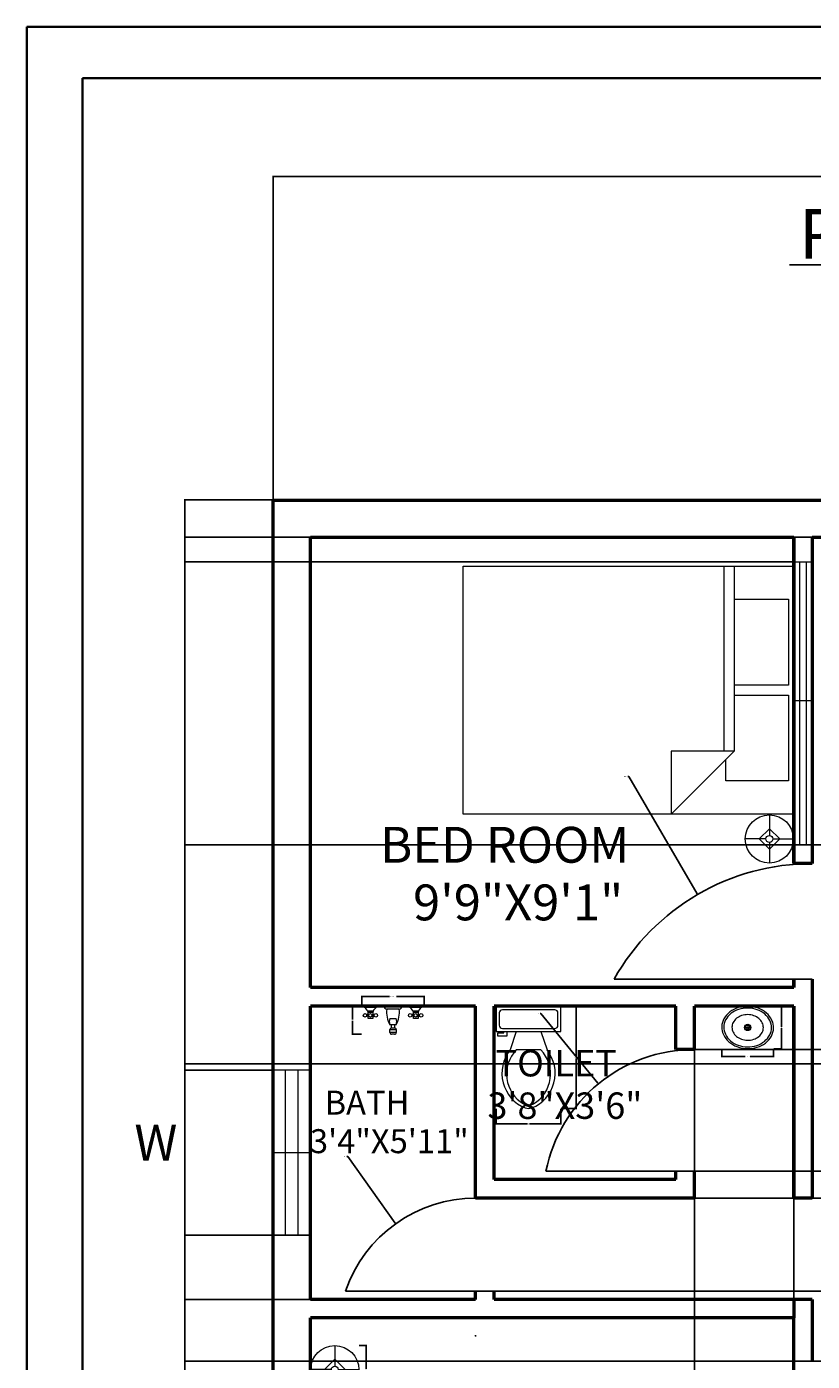
# Model space of a CAD drawing. Units: inches. Extents: x 1804 to 2221, y 1838 to 2403.
# Tile 2 of 3: x 1804 to 1995, y 2079 to 2403. Entities that reach past the tile are written whole.
import ezdxf

# ---------------------------------------------------------------- set-up
doc = ezdxf.new("R2010")
doc.units = ezdxf.units.IN
for name, color, linetype, lineweight in [('A-ANNO-DIMS', 2, 'Continuous', 18), ('A-ANNO-TEXT', 7, 'Continuous', 25), ('A-ANNO-TTLB', 7, 'Continuous', 35), ('A-AREA-IDEN', 7, 'Continuous', 25), ('A-DOOR', 3, 'Continuous', 25), ('A-FLOR-CASE', 8, 'Continuous', 25), ('A-FLOR-FIXT', 9, 'Continuous', 18), ('A-FLOR-STRS', 7, 'Continuous', 25), ('A-FURN', 8, 'Continuous', 18), ('A-GLAZ', 4, 'Continuous', 18), ('A-WALL', 7, 'Continuous', 50)]:
    doc.layers.add(name, color=color, linetype=linetype, lineweight=lineweight)
doc.styles.get("Standard").update_dxf_attribs({"font": 'arial.ttf'})
doc.dimstyles.get("Standard").update_dxf_attribs({"dimtxt": 0.18, "dimasz": 0.18, "dimexe": 0.18, "dimexo": 0.0625, "dimgap": 0.09, "dimtad": 0, "dimtih": 1, "dimtoh": 1, "dimdec": 4, "dimzin": 0, "dimdsep": 46, "dimtxsty": 'Standard', "dimcen": 0.09, "dimadec": 0, "dimazin": 0, "dimtfac": 1, "dimtdec": 4, "dimtofl": 0, "dimtmove": 0, "dimatfit": 3, "dimfxl": 1, "dimtolj": 1, "dimtzin": 0, "dimarcsym": 0})

# ---------------------------------------------------------------- blocks, each defined once
blk = doc.blocks.new('Bed - Queen')
for p, q in [((0, -80.00003), (0, 0)), ((0, 0), (59.99999, 0)), ((59.99999, 0), (59.99999, -80.00003)), ((7.99999, -1.2), (28.79998, -1.2)), ((7.99999, -14.4), (7.99999, -1.2)), ((28.79998, -1.2), (28.79998, -14.4)), ((31.19999, -1.2), (51.99999, -1.2)), ((31.19999, -14.4), (31.19999, -1.2)), ((51.99999, -1.2), (51.99999, -16.4)), ((0, -14.4), (44.8, -14.4)), ((59.99999, -29.6), (44.8, -14.4)), ((44.8, -14.4), (44.8, -29.6)), ((44.8, -16.8), (0, -16.8)), ((51.99999, -16.4), (46.79936, -16.4)), ((44.8, -29.6), (59.99999, -29.6)), ((59.99999, -80.00003), (0, -80.00003))]:
    blk.add_line(p, q)
blk = doc.blocks.new('Lamp - Table')
for p, q in [((0, 7), (0, 1)), ((-1, 0), (-7, 0)), ((0, 3), (-3, 0)), ((-3, 0), (0, -3)), ((3, 0), (0, 3)), ((0, -3), (3, 0)), ((1, 0), (7, 0)), ((0, -1), (0, -7))]:
    blk.add_line(p, q)
for radius in [7, 1]:
    blk.add_circle((0, 0), radius)
blk = doc.blocks.new('Toilet - top')
for p, q in [((9.5, -6), (9.5, -2)), ((-10, -8.5), (-8, -8.5)), ((-10, -9.5), (-10, -8.5)), ((-8, -8.5), (-8, -8)), ((-7, -8), (-7, -9.5)), ((-4, -8), (-6, -14)), ((4, -8), (6, -14)), ((-7, -9.5), (-10, -9.5)), ((4, -14), (-4, -14))]:
    blk.add_line(p, q)
blk.add_lwpolyline([(10.5, -8), (10.5, 0), (-10.5, 0), (-10.5, -8)], close=True)
for points in [[(-9.5, -2), (-9.5, -6)], [(8.5, -1), (-8.5, -1)], [(-8.5, -7), (8.5, -7)]]:
    blk.add_lwpolyline(points)
for centre, radius, start, end in [((-8.62, -1.88), 0.884, 81.8699, 188.1301), ((8.62, -1.88), 0.884, 351.8699, 98.1301), ((-8.62, -6.12), 0.884, 171.8699, 278.1301), ((8.62, -6.12), 0.884, 261.8699, 8.1301), ((3.52, -21.58), 12.17, 141.4691, 247.9714), ((4.2, -21.82), 11.33, 136.3677, 238.9468), ((-3.52, -21.58), 12.17, 292.0284, 38.5307), ((-4.2, -21.82), 11.33, 301.053, 43.6321), ((0, -27.88), 4, 245.7318, 294.2682), ((0, -29), 4, 254.8605, 285.1395)]:
    blk.add_arc(centre, radius, start, end)
blk = doc.blocks.new('Faucet - Bathroom front')
for p, q in [((-0.5, 4.25), (0.5, 4.25)), ((0.5, 3.75), (-0.5, 3.75)), ((-0.5, 3), (0.5, 3)), ((-0.25, 3), (-0.25, 3.5)), ((0.25, 3.5), (0.25, 3)), ((-5, 0), (-2.25, 0)), ((-4.5087, 0.25), (-2.7408, 0.25)), ((-4, 1.625), (-4.25, 1.625)), ((-4, 1.375), (-4.25, 1.375)), ((-3.1442, 0.75), (-4.0979, 0.75)), ((-3.25, 1.625), (-3, 1.625)), ((-3.25, 1.375), (-3, 1.375)), ((-1.5, 0), (1.5, 0)), ((-1, 0.5), (1, 0.5)), ((0.5, 2), (-0.5, 2)), ((2.25, 0), (5, 0)), ((2.7413, 0.25), (4.5092, 0.25)), ((3.25, 1.625), (3, 1.625)), ((3.25, 1.375), (3, 1.375)), ((4.1058, 0.75), (3.1521, 0.75)), ((4, 1.625), (4.25, 1.625)), ((4, 1.375), (4.25, 1.375))]:
    blk.add_line(p, q)
for points in [[(-0.25, 4.5), (0.25, 4.5)], [(-0.5, 3.75), (-0.5, 4.25)], [(0.25, 3.5), (-0.25, 3.5)], [(0.5, 4.25), (0.5, 3.75)]]:
    blk.add_lwpolyline(points)
for points in [[(-4, 1), (-4, 2), (-3.25, 2), (-3.25, 1)], [(3.25, 1), (3.25, 2), (4, 2), (4, 1)]]:
    blk.add_lwpolyline(points, close=True)
for centre in [(-4.5, 1.5), (-3.625, 1.5), (-2.75, 1.5), (2.75, 1.5), (3.625, 1.5), (4.5, 1.5)]:
    blk.add_circle(centre, 0.2795)
for centre, radius, start, end in [((-0.2575, 4.2575), 0.2426, 88.22243, 181.7776), ((0.2575, 4.2575), 0.2426, 358.2224, 91.77757), ((3, 1), 4.0311, 150.2551, 187.125), ((0.6413, 2.5), 1.246, 156.3417, 203.6583), ((-0.2575, 3.7425), 0.2426, 178.2224, 271.7776), ((0.2575, 3.7425), 0.2426, 268.2224, 1.777565), ((-3, 1), 4.0311, 352.875, 29.74488), ((-0.6413, 2.5), 1.246, 336.3417, 23.65835), ((-5.375, 1.375), 1.4252, 285.2551, 344.7449), ((-1.875, 1.375), 1.4252, 195.2551, 254.7449), ((-0.7962, -0.2038), 0.7327, 106.1502, 163.8498), ((0.7962, -0.2038), 0.7327, 16.1502, 73.84979), ((1.875, 1.375), 1.4252, 285.2551, 344.7449), ((5.375, 1.375), 1.4252, 195.2551, 254.7449)]:
    blk.add_arc(centre, radius, start, end)
blk = doc.blocks.new('Sink - Oval top')
for p, q in [((-1, 0), (1, 0)), ((0, 1), (0, -1))]:
    blk.add_line(p, q)
for points in [[(-12.23, 0.39, 0.117634), (-11.46, -3.36, 0.104469), (-8.88, -6.8, 0.090016), (-5.08, -9.07, 0.08192), (-0.32, -10.02, 0.08192), (4.49, -9.38, 0.090016), (8.42, -7.36, 0.104469), (11.22, -4.09, 0.117634), (12.23, -0.39, 0.117634), (11.46, 3.36, 0.104469), (8.88, 6.8, 0.090016), (5.08, 9.07, 0.08192), (0.32, 10.02, 0.08192), (-4.49, 9.38, 0.090016), (-8.42, 7.36, 0.104469), (-11.22, 4.09, 0.117634)], [(-11.29, 0.16, 0.118622), (-10.52, -3.25, 0.104678), (-8.07, -6.36, 0.089562), (-4.54, -8.37, 0.081185), (-0.13, -9.15, 0.081185), (4.3, -8.49, 0.089562), (7.89, -6.58, 0.104678), (10.42, -3.55, 0.118622), (11.29, -0.16, 0.118622), (10.52, 3.25, 0.104678), (8.07, 6.36, 0.089562), (4.54, 8.37, 0.081185), (0.13, 9.15, 0.081185), (-4.3, 8.49, 0.089562), (-7.89, 6.58, 0.104678), (-10.42, 3.55, 0.118622)], [(-7.42, 0.08, 0.118283), (-6.91, -2.17, 0.104607), (-5.29, -4.21, 0.089718), (-2.97, -5.53, 0.081436), (-0.07, -6.04, 0.081436), (2.84, -5.59, 0.089718), (5.2, -4.33, 0.104607), (6.86, -2.32, 0.118283), (7.42, -0.08, 0.118283), (6.91, 2.17, 0.104607), (5.29, 4.21, 0.089718), (2.97, 5.53, 0.081436), (0.07, 6.04, 0.081436), (-2.84, 5.59, 0.089718), (-5.2, 4.33, 0.104607), (-6.86, 2.32, 0.118283)]]:
    blk.add_lwpolyline(points, format="xyb", close=True)
for radius in [1.5, 1]:
    blk.add_circle((0, 0), radius)
blk = doc.blocks.new('*D13')
at = {"layer": 'A-ANNO-DIMS', "color": 0, "lineweight": -2, "transparency": 16777216}
for p, q in [((1884.89, 2083.28), (1886.75, 2083.28)), ((1886.57, 2083.1), (1886.57, 2077.63)), ((1886.57, 2071.8), (1886.57, 2077.27)), ((1884.89, 2071.62), (1886.75, 2071.62))]:
    blk.add_line(p, q, dxfattribs=at)
at = {"layer": 'A-ANNO-DIMS', "color": 0, "transparency": 16777216}
for points in [[(1886.54, 2083.1), (1886.6, 2083.1), (1886.57, 2083.28)], [(1886.54, 2071.8), (1886.6, 2071.8), (1886.57, 2071.62)]]:
    blk.add_solid(points, dxfattribs=at)
at = {"layer": 'Defpoints', "color": 0, "transparency": 16777216}
for p in [(1884.82, 2083.28), (1886.57, 2083.28), (1884.82, 2071.62)]:
    blk.add_point(p, dxfattribs=at)
at = {"layer": 'A-ANNO-DIMS', "color": 0, "transparency": 16777216, "insert": (1886.57, 2077.45), "char_height": 0.18, "attachment_point": 5}
blk.add_mtext('\\A1;12 TYP.', dxfattribs=at)
blk = doc.blocks.new('*D20')
at = {"layer": 'A-ANNO-DIMS', "color": 0, "lineweight": -2, "transparency": 16777216}
for p, q in [((1933.79, 2165.28), (1937.61, 2165.28)), ((1937.43, 2165.1), (1937.43, 2153.15)), ((1937.43, 2140.83), (1937.43, 2152.78)), ((1933.79, 2140.65), (1937.61, 2140.65))]:
    blk.add_line(p, q, dxfattribs=at)
at = {"layer": 'A-ANNO-DIMS', "color": 0, "transparency": 16777216}
for points in [[(1937.4, 2165.1), (1937.46, 2165.1), (1937.43, 2165.28)], [(1937.4, 2140.83), (1937.46, 2140.83), (1937.43, 2140.65)]]:
    blk.add_solid(points, dxfattribs=at)
at = {"layer": 'Defpoints', "color": 0, "transparency": 16777216}
for p in [(1933.73, 2165.28), (1937.43, 2165.28), (1933.73, 2140.65)]:
    blk.add_point(p, dxfattribs=at)
at = {"layer": 'A-ANNO-DIMS', "color": 0, "transparency": 16777216, "insert": (1937.43, 2152.97), "char_height": 0.18, "attachment_point": 5}
blk.add_mtext('\\A1;WC 25', dxfattribs=at)
blk = doc.blocks.new('*D21')
at = {"layer": 'A-ANNO-DIMS', "color": 0, "lineweight": -2, "transparency": 16777216}
for p, q in [((1918.08, 2140.59), (1918.08, 2136.78)), ((1933.73, 2140.59), (1933.73, 2136.78)), ((1918.26, 2136.96), (1925.69, 2136.96)), ((1933.55, 2136.96), (1926.11, 2136.96))]:
    blk.add_line(p, q, dxfattribs=at)
at = {"layer": 'A-ANNO-DIMS', "color": 0, "transparency": 16777216}
for points in [[(1918.26, 2136.99), (1918.26, 2136.93), (1918.08, 2136.96)], [(1933.55, 2136.99), (1933.55, 2136.93), (1933.73, 2136.96)]]:
    blk.add_solid(points, dxfattribs=at)
at = {"layer": 'Defpoints', "color": 0, "transparency": 16777216}
for p in [(1918.08, 2140.65), (1933.73, 2140.65), (1933.73, 2136.96)]:
    blk.add_point(p, dxfattribs=at)
at = {"layer": 'A-ANNO-DIMS', "color": 0, "transparency": 16777216, "insert": (1925.9, 2136.96), "char_height": 0.18, "attachment_point": 5}
blk.add_mtext('\\A1;16', dxfattribs=at)
blk = doc.blocks.new('*D22')
at = {"layer": 'A-ANNO-DIMS', "color": 0, "lineweight": -2, "transparency": 16777216}
for p, q in [((1885.54, 2165.53), (1885.54, 2167.92)), ((1900.66, 2165.53), (1900.66, 2167.92)), ((1885.72, 2167.74), (1892.24, 2167.74)), ((1900.48, 2167.74), (1893.97, 2167.74))]:
    blk.add_line(p, q, dxfattribs=at)
at = {"layer": 'A-ANNO-DIMS', "color": 0, "transparency": 16777216}
for points in [[(1885.72, 2167.77), (1885.72, 2167.71), (1885.54, 2167.74)], [(1900.48, 2167.77), (1900.48, 2167.71), (1900.66, 2167.74)]]:
    blk.add_solid(points, dxfattribs=at)
at = {"layer": 'Defpoints', "color": 0, "transparency": 16777216}
for p in [(1885.54, 2167.74), (1885.54, 2165.47), (1900.66, 2165.47)]:
    blk.add_point(p, dxfattribs=at)
at = {"layer": 'A-ANNO-DIMS', "color": 0, "transparency": 16777216, "insert": (1893.1, 2167.74), "char_height": 0.18, "attachment_point": 5}
blk.add_mtext('\\A1;BATH TAP 15', dxfattribs=at)
blk = doc.blocks.new('*D23')
at = {"layer": 'A-ANNO-DIMS', "color": 0, "lineweight": -2, "transparency": 16777216}
for p, q in [((1885.48, 2165.47), (1883.09, 2165.47)), ((1883.27, 2165.29), (1883.27, 2162.25)), ((1883.27, 2158.84), (1883.27, 2161.89)), ((1885.48, 2158.66), (1883.09, 2158.66))]:
    blk.add_line(p, q, dxfattribs=at)
at = {"layer": 'A-ANNO-DIMS', "color": 0, "transparency": 16777216}
for points in [[(1883.24, 2165.29), (1883.3, 2165.29), (1883.27, 2165.47)], [(1883.24, 2158.84), (1883.3, 2158.84), (1883.27, 2158.66)]]:
    blk.add_solid(points, dxfattribs=at)
at = {"layer": 'Defpoints', "color": 0, "transparency": 16777216}
for p in [(1885.54, 2165.47), (1883.27, 2158.66), (1885.54, 2158.66)]:
    blk.add_point(p, dxfattribs=at)
at = {"layer": 'A-ANNO-DIMS', "color": 0, "transparency": 16777216, "insert": (1883.27, 2162.07), "char_height": 0.18, "attachment_point": 5}
blk.add_mtext('\\A1;7', dxfattribs=at)
blk = doc.blocks.new('*D28')
at = {"layer": 'A-ANNO-DIMS', "color": 0, "lineweight": -2, "transparency": 16777216}
for p, q in [((1972.66, 2155.06), (1972.66, 2153.06)), ((1985.24, 2155.06), (1985.24, 2153.06)), ((1972.84, 2153.24), (1978.32, 2153.24)), ((1985.06, 2153.24), (1979.58, 2153.24))]:
    blk.add_line(p, q, dxfattribs=at)
at = {"layer": 'A-ANNO-DIMS', "color": 0, "transparency": 16777216}
for points in [[(1972.84, 2153.27), (1972.84, 2153.21), (1972.66, 2153.24)], [(1985.06, 2153.27), (1985.06, 2153.21), (1985.24, 2153.24)]]:
    blk.add_solid(points, dxfattribs=at)
at = {"layer": 'Defpoints', "color": 0, "transparency": 16777216}
for p in [(1972.66, 2155.13), (1985.24, 2155.13), (1985.24, 2153.24)]:
    blk.add_point(p, dxfattribs=at)
at = {"layer": 'A-ANNO-DIMS', "color": 0, "transparency": 16777216, "insert": (1978.95, 2153.24), "char_height": 0.18, "attachment_point": 5}
blk.add_mtext('\\A1;BASIN 13', dxfattribs=at)
blk = doc.blocks.new('*D29')
at = {"layer": 'A-ANNO-DIMS', "color": 0, "lineweight": -2, "transparency": 16777216}
for p, q in [((1985.31, 2165.45), (1987.31, 2165.45)), ((1987.13, 2165.27), (1987.13, 2160.47)), ((1987.13, 2155.31), (1987.13, 2160.1)), ((1985.31, 2155.13), (1987.31, 2155.13))]:
    blk.add_line(p, q, dxfattribs=at)
at = {"layer": 'A-ANNO-DIMS', "color": 0, "transparency": 16777216}
for points in [[(1987.1, 2165.27), (1987.16, 2165.27), (1987.13, 2165.45)], [(1987.1, 2155.31), (1987.16, 2155.31), (1987.13, 2155.13)]]:
    blk.add_solid(points, dxfattribs=at)
at = {"layer": 'Defpoints', "color": 0, "transparency": 16777216}
for p in [(1985.24, 2165.45), (1987.13, 2165.45), (1985.24, 2155.13)]:
    blk.add_point(p, dxfattribs=at)
at = {"layer": 'A-ANNO-DIMS', "color": 0, "transparency": 16777216, "insert": (1987.13, 2160.29), "char_height": 0.18, "attachment_point": 5}
blk.add_mtext('\\A1;10', dxfattribs=at)
blk = doc.blocks.new('*D32')
at = {"layer": 'A-ANNO-DIMS', "color": 0, "lineweight": -2, "transparency": 16777216}
for p, q in [((1864.1, 2288.03), (1864.1, 2366.45)), ((1864.28, 2366.27), (2016.31, 2366.27)), ((2168.92, 2366.27), (2016.89, 2366.27)), ((2169.1, 2288.03), (2169.1, 2366.45))]:
    blk.add_line(p, q, dxfattribs=at)
at = {"layer": 'A-ANNO-DIMS', "color": 0, "transparency": 16777216}
for points in [[(1864.28, 2366.3), (1864.28, 2366.24), (1864.1, 2366.27)], [(2168.92, 2366.3), (2168.92, 2366.24), (2169.1, 2366.27)]]:
    blk.add_solid(points, dxfattribs=at)
at = {"layer": 'Defpoints', "color": 0, "transparency": 16777216}
for p in [(2169.1, 2366.27), (1864.1, 2287.97), (2169.1, 2287.97)]:
    blk.add_point(p, dxfattribs=at)
at = {"layer": 'A-ANNO-DIMS', "color": 0, "transparency": 16777216, "insert": (2016.6, 2366.27), "char_height": 0.18, "attachment_point": 5}
blk.add_mtext('\\A1;305', dxfattribs=at)
blk = doc.blocks.new('*D33')
at = {"layer": 'A-ANNO-DIMS', "color": 0, "lineweight": -2, "transparency": 16777216}
for p, q in [((1864.04, 2287.97), (1842.52, 2287.97)), ((1842.7, 2287.79), (1842.7, 2123.65)), ((1842.7, 1959.15), (1842.7, 2123.29)), ((1864.04, 1958.97), (1842.52, 1958.97))]:
    blk.add_line(p, q, dxfattribs=at)
at = {"layer": 'A-ANNO-DIMS', "color": 0, "transparency": 16777216}
for points in [[(1842.67, 2287.79), (1842.73, 2287.79), (1842.7, 2287.97)], [(1842.67, 1959.15), (1842.73, 1959.15), (1842.7, 1958.97)]]:
    blk.add_solid(points, dxfattribs=at)
at = {"layer": 'Defpoints', "color": 0, "transparency": 16777216}
for p in [(1842.7, 2287.97), (1864.1, 2287.97), (1864.1, 1958.97)]:
    blk.add_point(p, dxfattribs=at)
at = {"layer": 'A-ANNO-DIMS', "color": 0, "transparency": 16777216, "insert": (1842.7, 2123.47), "char_height": 0.18, "attachment_point": 5}
blk.add_mtext('\\A1;329', dxfattribs=at)
blk = doc.blocks.new('*D34')
at = {"layer": 'A-ANNO-DIMS', "color": 0, "lineweight": -2, "transparency": 16777216}
for p, q in [((1990.04, 2272.97), (1842.52, 2272.97)), ((1842.7, 2272.79), (1842.7, 2238.9)), ((1842.7, 2204.65), (1842.7, 2238.54)), ((1990.04, 2204.47), (1842.52, 2204.47))]:
    blk.add_line(p, q, dxfattribs=at)
at = {"layer": 'A-ANNO-DIMS', "color": 0, "transparency": 16777216}
for points in [[(1842.67, 2272.79), (1842.73, 2272.79), (1842.7, 2272.97)], [(1842.67, 2204.65), (1842.73, 2204.65), (1842.7, 2204.47)]]:
    blk.add_solid(points, dxfattribs=at)
at = {"layer": 'Defpoints', "color": 0, "transparency": 16777216}
for p in [(1842.7, 2272.97), (1990.1, 2272.97), (1990.1, 2204.47)]:
    blk.add_point(p, dxfattribs=at)
at = {"layer": 'A-ANNO-DIMS', "color": 0, "transparency": 16777216, "insert": (1842.7, 2238.72), "char_height": 0.18, "attachment_point": 5}
blk.add_mtext('\\A1;68.5', dxfattribs=at)
blk = doc.blocks.new('*D39')
at = {"layer": 'A-ANNO-DIMS', "color": 0, "lineweight": -2, "transparency": 16777216}
for p, q in [((1873.04, 2109.97), (1842.52, 2109.97)), ((1842.7, 2109.79), (1842.7, 2102.4)), ((1842.7, 2094.65), (1842.7, 2102.04)), ((1873.04, 2094.47), (1842.52, 2094.47))]:
    blk.add_line(p, q, dxfattribs=at)
at = {"layer": 'A-ANNO-DIMS', "color": 0, "transparency": 16777216}
for points in [[(1842.67, 2109.79), (1842.73, 2109.79), (1842.7, 2109.97)], [(1842.67, 2094.65), (1842.73, 2094.65), (1842.7, 2094.47)]]:
    blk.add_solid(points, dxfattribs=at)
at = {"layer": 'Defpoints', "color": 0, "transparency": 16777216}
for p in [(1842.7, 2109.97), (1873.1, 2109.97), (1873.1, 2094.47)]:
    blk.add_point(p, dxfattribs=at)
at = {"layer": 'A-ANNO-DIMS', "color": 0, "transparency": 16777216, "insert": (1842.7, 2102.22), "char_height": 0.18, "attachment_point": 5}
blk.add_mtext('\\A1;15.5', dxfattribs=at)
blk = doc.blocks.new('*D40')
at = {"layer": 'A-ANNO-DIMS', "color": 0, "lineweight": -2, "transparency": 16777216}
for p, q in [((1864.04, 2149.97), (1842.52, 2149.97)), ((1842.7, 2149.79), (1842.7, 2130.15)), ((1842.7, 2110.15), (1842.7, 2129.79)), ((1864.04, 2109.97), (1842.52, 2109.97))]:
    blk.add_line(p, q, dxfattribs=at)
at = {"layer": 'A-ANNO-DIMS', "color": 0, "transparency": 16777216}
for points in [[(1842.67, 2149.79), (1842.73, 2149.79), (1842.7, 2149.97)], [(1842.67, 2110.15), (1842.73, 2110.15), (1842.7, 2109.97)]]:
    blk.add_solid(points, dxfattribs=at)
at = {"layer": 'Defpoints', "color": 0, "transparency": 16777216}
for p in [(1842.7, 2149.97), (1864.1, 2149.97), (1864.1, 2109.97)]:
    blk.add_point(p, dxfattribs=at)
at = {"layer": 'A-ANNO-DIMS', "color": 0, "transparency": 16777216, "insert": (1842.7, 2129.97), "char_height": 0.18, "attachment_point": 5}
blk.add_mtext('\\A1;40', dxfattribs=at)
blk = doc.blocks.new('*D43')
at = {"layer": 'A-ANNO-DIMS', "color": 0, "lineweight": -2, "transparency": 16777216}
for p, q in [((2030.54, 2278.97), (1842.52, 2278.97)), ((1842.7, 2278.79), (1842.7, 2241.9)), ((1842.7, 2204.65), (1842.7, 2241.54)), ((2030.54, 2204.47), (1842.52, 2204.47))]:
    blk.add_line(p, q, dxfattribs=at)
at = {"layer": 'A-ANNO-DIMS', "color": 0, "transparency": 16777216}
for points in [[(1842.67, 2278.79), (1842.73, 2278.79), (1842.7, 2278.97)], [(1842.67, 2204.65), (1842.73, 2204.65), (1842.7, 2204.47)]]:
    blk.add_solid(points, dxfattribs=at)
at = {"layer": 'Defpoints', "color": 0, "transparency": 16777216}
for p in [(1842.7, 2278.97), (2030.6, 2278.97), (2030.6, 2204.47)]:
    blk.add_point(p, dxfattribs=at)
at = {"layer": 'A-ANNO-DIMS', "color": 0, "transparency": 16777216, "insert": (1842.7, 2241.72), "char_height": 0.18, "attachment_point": 5}
blk.add_mtext('\\A1;74.5', dxfattribs=at)
blk = doc.blocks.new('*D48')
at = {"layer": 'A-ANNO-DIMS', "color": 0, "lineweight": -2, "transparency": 16777216}
for p, q in [((2140.04, 2151.47), (1842.52, 2151.47)), ((1842.7, 2151.29), (1842.7, 2115.65)), ((1842.7, 2079.65), (1842.7, 2115.29)), ((2052.04, 2079.47), (1842.52, 2079.47))]:
    blk.add_line(p, q, dxfattribs=at)
at = {"layer": 'A-ANNO-DIMS', "color": 0, "transparency": 16777216}
for points in [[(1842.67, 2151.29), (1842.73, 2151.29), (1842.7, 2151.47)], [(1842.67, 2079.65), (1842.73, 2079.65), (1842.7, 2079.47)]]:
    blk.add_solid(points, dxfattribs=at)
at = {"layer": 'Defpoints', "color": 0, "transparency": 16777216}
for p in [(1842.7, 2151.47), (2140.1, 2151.47), (2052.1, 2079.47)]:
    blk.add_point(p, dxfattribs=at)
at = {"layer": 'A-ANNO-DIMS', "color": 0, "transparency": 16777216, "insert": (1842.7, 2115.47), "char_height": 0.18, "attachment_point": 5}
blk.add_mtext('\\A1;72', dxfattribs=at)
blk = doc.blocks.new('*D51')
at = {"layer": 'A-ANNO-DIMS', "color": 0, "lineweight": -2, "transparency": 16777216}
for p, q in [((1913.16, 2118.97), (2190.68, 2118.97)), ((2190.5, 2118.79), (2190.5, 2107.9)), ((2190.5, 2096.65), (2190.5, 2107.54)), ((1913.16, 2096.47), (2190.68, 2096.47))]:
    blk.add_line(p, q, dxfattribs=at)
at = {"layer": 'A-ANNO-DIMS', "color": 0, "transparency": 16777216}
for points in [[(2190.47, 2118.79), (2190.53, 2118.79), (2190.5, 2118.97)], [(2190.47, 2096.65), (2190.53, 2096.65), (2190.5, 2096.47)]]:
    blk.add_solid(points, dxfattribs=at)
at = {"layer": 'Defpoints', "color": 0, "transparency": 16777216}
for p in [(1913.1, 2118.97), (2190.5, 2118.97), (1913.1, 2096.47)]:
    blk.add_point(p, dxfattribs=at)
at = {"layer": 'A-ANNO-DIMS', "color": 0, "transparency": 16777216, "insert": (2190.5, 2107.72), "char_height": 0.18, "attachment_point": 5}
blk.add_mtext('\\A1;22.5', dxfattribs=at)
blk = doc.blocks.new('*D52')
at = {"layer": 'A-ANNO-DIMS', "color": 0, "lineweight": -2, "transparency": 16777216}
for p, q in [((1966.16, 2154.97), (2190.68, 2154.97)), ((2190.5, 2154.79), (2190.5, 2140.4)), ((2190.5, 2125.65), (2190.5, 2140.04)), ((1966.16, 2125.47), (2190.68, 2125.47))]:
    blk.add_line(p, q, dxfattribs=at)
at = {"layer": 'A-ANNO-DIMS', "color": 0, "transparency": 16777216}
for points in [[(2190.47, 2154.79), (2190.53, 2154.79), (2190.5, 2154.97)], [(2190.47, 2125.65), (2190.53, 2125.65), (2190.5, 2125.47)]]:
    blk.add_solid(points, dxfattribs=at)
at = {"layer": 'Defpoints', "color": 0, "transparency": 16777216}
for p in [(1966.1, 2154.97), (2190.5, 2154.97), (1966.1, 2125.47)]:
    blk.add_point(p, dxfattribs=at)
at = {"layer": 'A-ANNO-DIMS', "color": 0, "transparency": 16777216, "insert": (2190.5, 2140.22), "char_height": 0.18, "attachment_point": 5}
blk.add_mtext('\\A1;29.5', dxfattribs=at)
blk = doc.blocks.new('*D59')
at = {"layer": 'A-ANNO-DIMS', "color": 0, "lineweight": -2, "transparency": 16777216}
for p, q in [((1966.1, 2154.91), (1966.1, 1937.39)), ((1990.1, 2154.91), (1990.1, 1937.39)), ((1966.28, 1937.57), (1977.88, 1937.57)), ((1989.92, 1937.57), (1978.32, 1937.57))]:
    blk.add_line(p, q, dxfattribs=at)
at = {"layer": 'A-ANNO-DIMS', "color": 0, "transparency": 16777216}
for points in [[(1966.28, 1937.6), (1966.28, 1937.54), (1966.1, 1937.57)], [(1989.92, 1937.6), (1989.92, 1937.54), (1990.1, 1937.57)]]:
    blk.add_solid(points, dxfattribs=at)
at = {"layer": 'Defpoints', "color": 0, "transparency": 16777216}
for p in [(1966.1, 2154.97), (1990.1, 2154.97), (1990.1, 1937.57)]:
    blk.add_point(p, dxfattribs=at)
at = {"layer": 'A-ANNO-DIMS', "color": 0, "transparency": 16777216, "insert": (1978.1, 1937.57), "char_height": 0.18, "attachment_point": 5}
blk.add_mtext('\\A1;24', dxfattribs=at)
blk = doc.blocks.new('*D60')
at = {"layer": 'A-ANNO-DIMS', "color": 0, "lineweight": -2, "transparency": 16777216}
for p, q in [((1949.97, 2221.04), (1950.15, 2221.04)), ((1950.15, 2221.04), (1966.73, 2192.61)), ((1994.51, 2144.83), (1994.69, 2144.83)), ((1994.6, 2144.74), (1994.6, 2144.92))]:
    blk.add_line(p, q, dxfattribs=at)
at = {"layer": 'A-ANNO-DIMS', "color": 0, "transparency": 16777216}
blk.add_solid([(1966.75, 2192.63), (1966.7, 2192.6), (1966.82, 2192.46)], dxfattribs=at)
at = {"layer": 'Defpoints', "color": 0, "transparency": 16777216}
for p in [(1966.82, 2192.46), (1994.6, 2144.83)]:
    blk.add_point(p, dxfattribs=at)
at = {"layer": 'A-ANNO-DIMS', "color": 0, "transparency": 16777216, "insert": (1949.49, 2221.04), "char_height": 0.18, "attachment_point": 5}
blk.add_mtext('\\A1;R55.14', dxfattribs=at)
blk = doc.blocks.new('*D62')
at = {"layer": 'A-ANNO-DIMS', "color": 0, "lineweight": -2, "transparency": 16777216}
for p, q in [((1928.69, 2163.69), (1928.87, 2163.69)), ((1928.87, 2163.69), (1942.71, 2146.79)), ((1966.01, 2118.25), (1966.19, 2118.25)), ((1966.1, 2118.16), (1966.1, 2118.34))]:
    blk.add_line(p, q, dxfattribs=at)
at = {"layer": 'A-ANNO-DIMS', "color": 0, "transparency": 16777216}
blk.add_solid([(1942.74, 2146.81), (1942.69, 2146.77), (1942.83, 2146.65)], dxfattribs=at)
at = {"layer": 'Defpoints', "color": 0, "transparency": 16777216}
for p in [(1942.83, 2146.65), (1966.1, 2118.25)]:
    blk.add_point(p, dxfattribs=at)
at = {"layer": 'A-ANNO-DIMS', "color": 0, "transparency": 16777216, "insert": (1928.14, 2163.69), "char_height": 0.18, "attachment_point": 5}
blk.add_mtext('\\A1;R36.716', dxfattribs=at)
blk = doc.blocks.new('*D63')
at = {"layer": 'A-ANNO-DIMS', "color": 0, "lineweight": -2, "transparency": 16777216}
for p, q in [((1881.95, 2129.02), (1882.13, 2129.02)), ((1882.13, 2129.02), (1893.64, 2112.91)), ((1913.01, 2085.67), (1913.19, 2085.67)), ((1913.1, 2085.58), (1913.1, 2085.76))]:
    blk.add_line(p, q, dxfattribs=at)
at = {"layer": 'A-ANNO-DIMS', "color": 0, "transparency": 16777216}
blk.add_solid([(1893.67, 2112.93), (1893.62, 2112.89), (1893.75, 2112.77)], dxfattribs=at)
at = {"layer": 'Defpoints', "color": 0, "transparency": 16777216}
for p in [(1893.75, 2112.77), (1913.1, 2085.67)]:
    blk.add_point(p, dxfattribs=at)
at = {"layer": 'A-ANNO-DIMS', "color": 0, "transparency": 16777216, "insert": (1881.54, 2129.02), "char_height": 0.18, "attachment_point": 5}
blk.add_mtext('\\A1;R33.3', dxfattribs=at)

msp = doc.modelspace()

# ---------------------------------------------------------------- linework, layer by layer
at = {"layer": 'A-ANNO-TEXT'}
msp.add_line((1989.0457, 2344.8659), (2036.3709, 2344.8659), dxfattribs=at)
at = {"layer": 'A-ANNO-TTLB'}
for points in [[(1804.4104, 2402.5437), (2220.7086, 2402.5437), (2220.7086, 1837.8762), (1804.4104, 1837.8762)], [(1817.9401, 2390.0649), (2205.0975, 2390.0649), (2205.0975, 1852.4349), (1817.9401, 1852.4349)]]:
    msp.add_lwpolyline(points, close=True, dxfattribs=at)
at = {"layer": 'A-DOOR'}
for p, q in [((1994.6006, 2171.9683), (1946.6006, 2171.9683)), ((1966.1006, 2125.4683), (1930.1006, 2125.4683)), ((1917.6006, 2096.4683), (1881.6006, 2096.4683))]:
    msp.add_line(p, q, dxfattribs=at)
for centre, radius, end in [((1994.6006, 2144.8254), 55.1429, 150.512874), ((1966.1006, 2118.2522), 36.7161, 168.665429), ((1913.1006, 2085.6683), 33.3, 161.075356)]:
    msp.add_arc(centre, radius, 90, end, dxfattribs=at)
at = {"layer": 'A-FLOR-CASE'}
msp.add_line((1966.1006, 2154.9683), (1990.1006, 2154.9683), dxfattribs=at)
at = {"layer": 'A-FLOR-STRS'}
msp.add_line((1994.6006, 2204.4683), (2132.6006, 2204.4683), dxfattribs=at)
at = {"layer": 'A-GLAZ'}
for p, q in [((1990.1006, 2272.9683), (1994.6006, 2272.9683)), ((1991.6006, 2204.4683), (1991.6006, 2272.9683)), ((1993.1006, 2272.9683), (1993.1006, 2204.4683)), ((1990.1006, 2239.4683), (1994.6006, 2239.4683)), ((1994.6006, 2204.4683), (1990.1006, 2204.4683)), ((1873.1006, 2149.9683), (1864.1006, 2149.9683)), ((1867.1006, 2109.9683), (1867.1006, 2149.9683)), ((1870.1006, 2109.9683), (1870.1006, 2149.9683)), ((1873.1006, 2129.9683), (1864.1006, 2129.9683)), ((1873.1006, 2109.9683), (1864.1006, 2109.9683))]:
    msp.add_line(p, q, dxfattribs=at)
at = {"layer": 'A-WALL'}
for p, q in [((1864.1006, 2287.9683), (2169.1006, 2287.9683)), ((1864.1006, 2169.9683), (1864.1006, 2287.9683)), ((1864.1006, 1958.9683), (1864.1006, 2278.9683)), ((1873.1006, 2278.9683), (1990.1006, 2278.9683)), ((1873.1006, 2169.9683), (1873.1006, 2278.9683)), ((1990.1006, 2278.9683), (1990.1006, 2199.9683)), ((1990.1006, 2199.9683), (1990.1006, 2278.9683)), ((1994.6006, 2278.9683), (1994.6006, 2204.4683)), ((1994.6006, 2278.9683), (1994.6006, 2213.4683)), ((1994.6006, 2278.9683), (2160.1006, 2278.9683)), ((1994.6006, 2204.4683), (1994.6006, 2199.9683)), ((1994.6006, 2204.4683), (1994.6006, 2199.9683)), ((1994.6006, 2199.9683), (1990.1006, 2199.9683)), ((1990.1006, 2171.9683), (1990.1006, 2169.9683)), ((1990.1006, 2169.9683), (1990.1006, 2171.9683)), ((1994.6006, 2171.9683), (1994.6006, 2169.9683)), ((1994.6006, 2171.9683), (1994.6006, 2118.9683)), ((1990.1006, 2169.9683), (1873.1006, 2169.9683)), ((1873.1006, 2094.4683), (1873.1006, 2165.4683)), ((1913.1006, 2165.4683), (1873.1006, 2165.4683)), ((1913.1006, 2118.9683), (1913.1006, 2165.4683)), ((1917.6006, 2123.4683), (1917.6006, 2165.4683)), ((1961.6006, 2165.4683), (1917.6006, 2165.4683)), ((1961.6006, 2154.9683), (1961.6006, 2165.4683)), ((1990.1006, 2165.4683), (1966.1006, 2165.4683)), ((1966.1006, 2154.9683), (1966.1006, 2165.4683)), ((1990.1006, 2118.9683), (1990.1006, 2165.4683)), ((1990.1006, 2165.4683), (1990.1006, 2118.9683)), ((1966.1006, 2154.9683), (1961.6006, 2154.9683)), ((1961.6006, 2123.4683), (1917.6006, 2123.4683)), ((1961.6006, 2123.4683), (1961.6006, 2125.4683)), ((1966.1006, 2118.9683), (1966.1006, 2125.4683)), ((1966.1006, 2118.9683), (1913.1006, 2118.9683)), ((1994.6006, 2118.9683), (1990.1006, 2118.9683)), ((1913.1006, 2094.4683), (1873.1006, 2094.4683)), ((1913.1006, 2094.4683), (1913.1006, 2096.4683)), ((1917.6006, 2094.4683), (1917.6006, 2096.4683)), ((1994.6006, 2094.4683), (1917.6006, 2094.4683)), ((1990.1006, 2094.4683), (1990.1006, 2089.9683)), ((1994.6006, 2094.4683), (1994.6006, 2089.9683)), ((1994.6006, 2094.4683), (1994.6006, 2079.4683)), ((1873.1006, 1967.9683), (1873.1006, 2089.9683)), ((1990.1006, 2089.9683), (1873.1006, 2089.9683)), ((1990.1006, 2000.9683), (1990.1006, 2089.9683))]:
    msp.add_line(p, q, dxfattribs=at)

# ---------------------------------------------------------------- block references
at = {"layer": 'A-FLOR-FIXT', "xscale": 1.511751829720732, "yscale": 1.511751829720732, "zscale": 1.511751829720732, "rotation": 180}
msp.add_blockref('Faucet - Bathroom front', (1893.1006, 2165.4683), dxfattribs=at)
at = {"layer": 'A-FLOR-FIXT'}
for name, p, xscale, yscale, zscale in [('Toilet - top', (1925.9044, 2165.283), 0.7453567138886626, 0.7453567138886626, 0.7453567138886626), ('Sink - Oval top', (1978.9519, 2160.2868), 0.5124705556322554, 0.5124705556322554, 0.5124705556322554)]:
    msp.add_blockref(name, p, dxfattribs=dict(at, xscale=xscale, yscale=yscale, zscale=zscale))
at = {"layer": 'A-FURN', "rotation": 270}
msp.add_blockref('Bed - Queen', (1990.0635, 2271.9465), dxfattribs=at)
at = {"layer": 'A-FURN', "xscale": 0.8325724254019075, "yscale": 0.8325724254019075, "zscale": 0.8325724254019075}
for p in [(1984.2041, 2205.9067), (1878.9968, 2077.4528)]:
    msp.add_blockref('Lamp - Table', p, dxfattribs=at)

# ---------------------------------------------------------------- texts
at = {"layer": 'A-ANNO-TEXT'}
for s, height, p in [('PLAN', 12, (1991.349, 2346.384)), ('                     W', 8.682741, (1774.7672, 2128.0764))]:
    msp.add_text(s, height=height, dxfattribs=at).set_placement(p)
at = {"layer": 'A-AREA-IDEN'}
for s, height, p in [('BED ROOM', 8.68274, (1889.9768, 2200.1582)), ('   9\'9"X9\'1"', 8.682741, (1889.9768, 2186.2102)), ('    TOILET', 6.39827, (1910.0848, 2148.4307)), ('         BATH', 5.808884, (1860.5526, 2139.1829)), ('   3\'8"X3\'6"', 6.398267, (1910.0848, 2138.1525)), ('       3\'4"X5\'11"', 5.808884, (1860.5526, 2129.8514))]:
    msp.add_text(s, height=height, dxfattribs=at).set_placement(p)

# ---------------------------------------------------------------- dimensions: what is measured, and where the dimension line sits
at = {"layer": 'A-ANNO-DIMS'}
for base, p1, p2, picture, middle in [((2169.1006, 2366.2659), (1864.1006, 2287.9683), (2169.1006, 2287.9683), '*D32', (2016.6006, 2366.2659)), ((1990.1006, 1937.5683), (1966.1006, 2154.9683), (1990.1006, 2154.9683), '*D59', (1978.1006, 1937.5683)), ((1933.7307, 2136.9571), (1918.0782, 2140.6518), (1933.7307, 2140.6518), '*D21', (1925.9044, 2136.9571))]:
    dim = msp.add_linear_dim(base=base, p1=p1, p2=p2, dimstyle='Standard', override={"dimdec": 0, "dimlfac": 1, "dimrnd": 0, "dimzin": 0, "dimdsep": 46, "dimlunit": 2}, dxfattribs=at)
    dim.commit()
    dim.dimension.update_dxf_attribs({"geometry": picture, "text_midpoint": middle})
for base, p1, p2, angle, override, picture, middle in [((1842.7006, 2287.9683), (1864.1006, 1958.9683), (1864.1006, 2287.9683), 90, {"dimdec": 0, "dimlfac": 1, "dimrnd": 0, "dimzin": 0, "dimdsep": 46, "dimlunit": 2}, '*D33', (1842.7006, 2123.4683)), ((1842.7006, 2278.9683), (2030.6006, 2204.4683), (2030.6006, 2278.9683), 90, {"dimdec": 1, "dimlfac": 1, "dimrnd": 0, "dimzin": 0, "dimdsep": 46, "dimlunit": 2}, '*D43', (1842.7006, 2241.7183)), ((1842.7006, 2272.9683), (1990.1006, 2204.4683), (1990.1006, 2272.9683), 90, {"dimdec": 1, "dimlfac": 1, "dimrnd": 0, "dimzin": 0, "dimdsep": 46, "dimlunit": 2}, '*D34', (1842.7006, 2238.7183)), ((1883.2742, 2158.6623), (1885.5418, 2165.4683), (1885.5418, 2158.6623), 270, {"dimdec": 0, "dimlfac": 1, "dimrnd": 0, "dimzin": 0, "dimdsep": 46, "dimlunit": 2}, '*D23', (1883.2742, 2162.0653)), ((1987.1299, 2165.4466), (1985.2427, 2155.1271), (1985.2427, 2165.4466), 90, {"dimdec": 0, "dimlfac": 1, "dimrnd": 0, "dimzin": 0, "dimdsep": 46, "dimlunit": 2}, '*D29', (1987.1299, 2160.2868)), ((2190.5006, 2154.9683), (1966.1006, 2125.4683), (1966.1006, 2154.9683), 90, {"dimdec": 1, "dimlfac": 1, "dimrnd": 0, "dimzin": 0, "dimdsep": 46, "dimlunit": 2}, '*D52', (2190.5006, 2140.2183)), ((1842.7006, 2151.4683), (2052.1006, 2079.4683), (2140.1006, 2151.4683), 90, {"dimdec": 0, "dimlfac": 1, "dimrnd": 0, "dimzin": 0, "dimdsep": 46, "dimlunit": 2}, '*D48', (1842.7006, 2115.4683)), ((1842.7006, 2149.9683), (1864.1006, 2109.9683), (1864.1006, 2149.9683), 90, {"dimdec": 0, "dimlfac": 1, "dimrnd": 0, "dimzin": 0, "dimdsep": 46, "dimlunit": 2}, '*D40', (1842.7006, 2129.9683)), ((2190.5006, 2118.9683), (1913.1006, 2096.4683), (1913.1006, 2118.9683), 90, {"dimdec": 1, "dimlfac": 1, "dimrnd": 0, "dimzin": 0, "dimdsep": 46, "dimlunit": 2}, '*D51', (2190.5006, 2107.7183)), ((1842.7006, 2109.9683), (1873.1006, 2094.4683), (1873.1006, 2109.9683), 90, {"dimdec": 1, "dimlfac": 1, "dimrnd": 0, "dimzin": 0, "dimdsep": 46, "dimlunit": 2}, '*D39', (1842.7006, 2102.2183))]:
    dim = msp.add_linear_dim(base=base, p1=p1, p2=p2, angle=angle, dimstyle='Standard', override=override, dxfattribs=at)
    dim.commit()
    dim.dimension.update_dxf_attribs({"geometry": picture, "text_midpoint": middle})
for center, mpoint, override, picture, middle in [((1994.6006, 2144.8254), (1966.8161, 2192.4569), {"dimdec": 2, "dimlfac": 1, "dimrnd": 0, "dimzin": 0, "dimdsep": 46, "dimlunit": 2}, '*D60', (1949.4859, 2221.0357)), ((1966.1006, 2118.2522), (1942.8289, 2146.6511), {"dimdec": 3, "dimlfac": 1, "dimrnd": 0, "dimzin": 0, "dimdsep": 46, "dimlunit": 2}, '*D62', (1928.1362, 2163.6905)), ((1913.1006, 2085.6683), (1893.7453, 2112.7656), {"dimdec": 1, "dimlfac": 1, "dimrnd": 0, "dimzin": 0, "dimdsep": 46, "dimlunit": 2}, '*D63', (1881.5422, 2129.0239))]:
    dim = msp.add_radius_dim(center=center, mpoint=mpoint, dimstyle='Standard', override=override, dxfattribs=at)
    dim.commit()
    dim.dimension.update_dxf_attribs({"geometry": picture, "text_midpoint": middle, "dimtype": 164})
for base, p1, p2, angle, text, picture, middle in [((1885.5418, 2167.7359), (1900.6594, 2165.4683), (1885.5418, 2165.4683), 180, 'BATH TAP <>', '*D22', (1893.1006, 2167.7359)), ((1937.4254, 2165.283), (1933.7307, 2140.6518), (1933.7307, 2165.283), 90, 'WC <>', '*D20', (1937.4254, 2152.9674)), ((1886.5733, 2083.2808), (1884.8249, 2071.6248), (1884.8249, 2083.2808), 90, '<> TYP.', '*D13', (1886.5733, 2077.4528))]:
    dim = msp.add_linear_dim(base=base, p1=p1, p2=p2, angle=angle, text=text, dimstyle='Standard', override={"dimdec": 0, "dimlfac": 1, "dimrnd": 0, "dimzin": 0, "dimdsep": 46, "dimlunit": 2}, dxfattribs=at)
    dim.commit()
    dim.dimension.update_dxf_attribs({"geometry": picture, "text_midpoint": middle})
dim = msp.add_linear_dim(base=(1985.2427, 2153.2399), p1=(1972.6611, 2155.1271), p2=(1985.2427, 2155.1271), text='BASIN <>', dimstyle='Standard', override={"dimdec": 0, "dimlfac": 1, "dimrnd": 0, "dimzin": 0, "dimdsep": 46, "dimlunit": 2}, dxfattribs=at)
dim.commit()
dim.dimension.update_dxf_attribs({"geometry": '*D28', "text_midpoint": (1978.9519, 2153.2399)})

doc.saveas('drawing.dxf')
